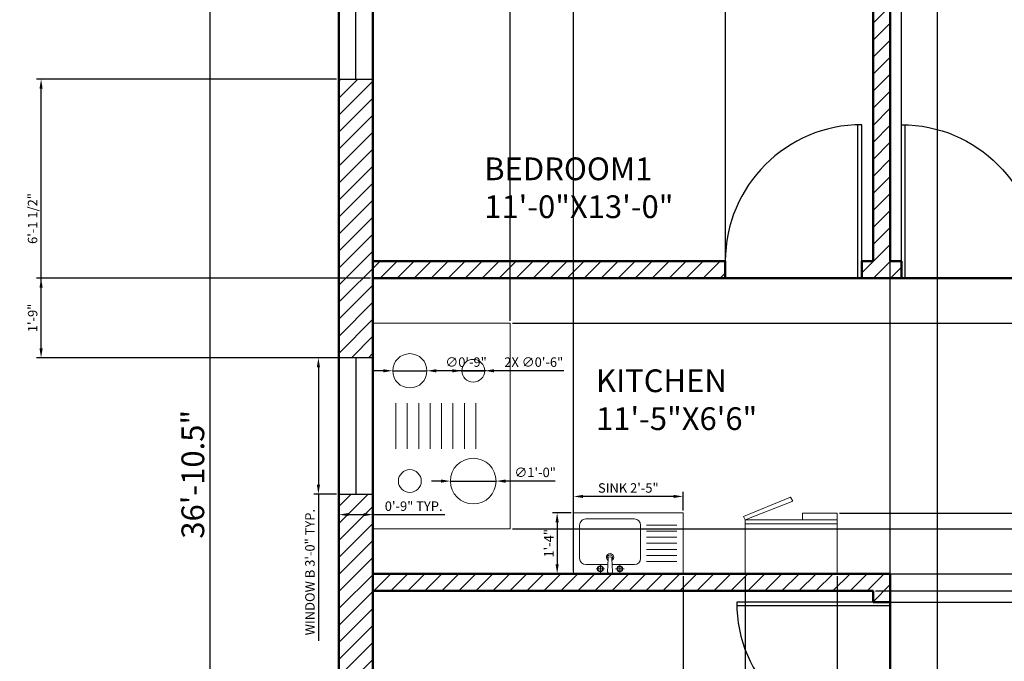
# Model space of a CAD drawing. Units: inches. Extents: x 3064 to 3516, y 2736 to 3280.
# Tile 3 of 5: x 3064 to 3324, y 2941 to 3110. Entities that reach past the tile are written whole.
import ezdxf

# ---------------------------------------------------------------- set-up
doc = ezdxf.new("R2010")
doc.units = ezdxf.units.IN
for name, color, linetype, lineweight in [('A-ANNO-DIMS', 2, 'Continuous', 18), ('A-AREA-IDEN', 6, 'Continuous', 25), ('A-DOOR', 3, 'Continuous', 25), ('A-EQPM', 8, 'Continuous', 18), ('A-FLOR-FIXT', 9, 'Continuous', 20), ('A-GLAZ', 5, 'Continuous', 25), ('A-WALL', 7, 'Continuous', 50), ('A-WALL-PATT', 8, 'Continuous', 13)]:
    doc.layers.add(name, color=color, linetype=linetype, lineweight=lineweight)
doc.styles.get("Standard").update_dxf_attribs({"font": 'arial.ttf'})
doc.dimstyles.new('ISO-25', dxfattribs={"dimtxt": 2.5, "dimasz": 2.5, "dimexe": 1.25, "dimexo": 0.625, "dimtad": 1, "dimlunit": 3, "dimtxsty": 'Standard', "dimcen": 2.5, "dimadec": 0, "dimazin": 0, "dimtfac": 1, "dimtmove": 0, "dimatfit": 3, "dimfxl": 1, "dimarcsym": 0})

# ---------------------------------------------------------------- blocks, each defined once
blk = doc.blocks.new('*D4')
at = {"layer": 'A-ANNO-DIMS', "color": 0, "lineweight": -2, "transparency": 16777216}
for p, q in [((3147.27, 3211.51), (3112.57, 3211.51)), ((3113.82, 3209.01), (3113.82, 2771.51)), ((3147.27, 2769.01), (3112.57, 2769.01))]:
    blk.add_line(p, q, dxfattribs=at)
at = {"layer": 'A-ANNO-DIMS', "color": 0, "transparency": 16777216}
for points in [[(3113.4, 3209.01), (3114.23, 3209.01), (3113.82, 3211.51)], [(3113.4, 2771.51), (3114.23, 2771.51), (3113.82, 2769.01)]]:
    blk.add_solid(points, dxfattribs=at)
at = {"layer": 'Defpoints', "color": 0, "transparency": 16777216}
for p in [(3147.9, 3211.51), (3113.82, 2769.01), (3147.9, 2769.01)]:
    blk.add_point(p, dxfattribs=at)
at = {"layer": 'A-ANNO-DIMS', "color": 0, "transparency": 16777216, "insert": (3110.13, 2990.26), "char_height": 6, "attachment_point": 5, "rotation": 90}
blk.add_mtext('36\'-10.5"', dxfattribs=at)
blk = doc.blocks.new('kitchen sink8')
at = {"color": 0}
for p, q in [((0, 0), (-1080, 0)), ((-1080, 0), (-1080, -600)), ((0, -600), (0, 0)), ((-379.8, -90), (-600, -90)), ((-498, -48), (-414, -48)), ((-456, -6), (-456, -90)), ((-377.9, -151.2), (-384.1, -17.1)), ((-335.9, -17.1), (-342.1, -151.2)), ((-120, -90), (-340.2, -90)), ((-222, -48), (-306, -48)), ((-264, -6), (-264, -90)), ((-1020, -120), (-720, -120)), ((-1020, -180), (-720, -180)), ((-660, -150), (-660, -480)), ((-60, -480), (-60, -150)), ((-1020, -240), (-720, -240)), ((-1020, -300), (-720, -300)), ((-1020, -360), (-720, -360)), ((-1020, -420), (-720, -420)), ((-1020, -480), (-720, -480)), ((-600, -540), (-120, -540)), ((-1080, -600), (0, -600))]:
    blk.add_line(p, q, dxfattribs=at)
for centre, radius in [((-456, -48), 30), ((-456, -48), 24), ((-264, -48), 30), ((-264, -48), 24)]:
    blk.add_circle(centre, radius, dxfattribs=at)
for centre, radius, start, end in [((-360, -25.5), 25.5, 19.33284, 160.66716), ((-600, -150), 60, 90, 180), ((-120, -150), 60, 0, 90), ((-360, -162), 36, 121.86593, 58.13407), ((-360, -162), 24, 139.21522, 40.78479), ((-360, -149.3), 18, 186.0661, 353.9339), ((-600, -480), 60, 180, 270), ((-120, -480), 60, 270, 0)]:
    blk.add_arc(centre, radius, start, end, dxfattribs=at)
blk = doc.blocks.new('DOOR-SWING-36IN')
for p, q in [((-1, -4.5), (-1, 36)), ((0, 0), (0, 36))]:
    blk.add_line(p, q)
blk.add_arc((0, 0), 36, 90, 180)
blk = doc.blocks.new('WIN-60IN')
for p, q in [((0, 60), (0, 0)), ((9, 60), (0, 60)), ((4.5, 60), (4.5, 0)), ((9, 0), (9, 60)), ((0, 0), (9, 0))]:
    blk.add_line(p, q)
blk = doc.blocks.new('WIN-36IN')
for p, q in [((36, 9), (0, 9)), ((0, 9), (0, 0)), ((36, 0), (36, 9)), ((0, 4.5), (36, 4.5)), ((0, 0), (36, 0))]:
    blk.add_line(p, q)
blk = doc.blocks.new('*D21')
at = {"layer": 'A-ANNO-DIMS', "color": 0, "lineweight": -2, "transparency": 16777216}
for p, q in [((3147.27, 3021.01), (3141.25, 3021.01)), ((3142.5, 3018.51), (3142.5, 2987.51)), ((3147.27, 2985.01), (3141.25, 2985.01)), ((3142.5, 2985.01), (3142.5, 2946.33))]:
    blk.add_line(p, q, dxfattribs=at)
at = {"layer": 'A-ANNO-DIMS', "color": 0, "transparency": 16777216}
for points in [[(3142.08, 3018.51), (3142.91, 3018.51), (3142.5, 3021.01)], [(3142.08, 2987.51), (3142.91, 2987.51), (3142.5, 2985.01)]]:
    blk.add_solid(points, dxfattribs=at)
at = {"layer": 'Defpoints', "color": 0, "transparency": 16777216}
for p in [(3147.9, 3021.01), (3142.5, 2985.01), (3147.9, 2985.01)]:
    blk.add_point(p, dxfattribs=at)
at = {"layer": 'A-ANNO-DIMS', "color": 0, "transparency": 16777216, "insert": (3140.58, 2964.42), "char_height": 2.5, "attachment_point": 5, "rotation": 90}
blk.add_mtext('WINDOW B 3\'-0" TYP.', dxfattribs=at)
blk = doc.blocks.new('*D22')
at = {"layer": 'A-ANNO-DIMS', "color": 0, "lineweight": -2, "transparency": 16777216}
for p, q in [((3147.9, 2984.39), (3147.9, 2978.36)), ((3156.9, 2984.39), (3156.9, 2978.36)), ((3150.4, 2979.61), (3154.4, 2979.61)), ((3156.9, 2979.61), (3175.89, 2979.61))]:
    blk.add_line(p, q, dxfattribs=at)
at = {"layer": 'A-ANNO-DIMS', "color": 0, "transparency": 16777216}
for points in [[(3150.4, 2980.03), (3150.4, 2979.2), (3147.9, 2979.61)], [(3154.4, 2980.03), (3154.4, 2979.2), (3156.9, 2979.61)]]:
    blk.add_solid(points, dxfattribs=at)
at = {"layer": 'Defpoints', "color": 0, "transparency": 16777216}
for p in [(3147.9, 2985.01), (3156.9, 2985.01), (3156.9, 2979.61)]:
    blk.add_point(p, dxfattribs=at)
at = {"layer": 'A-ANNO-DIMS', "color": 0, "transparency": 16777216, "insert": (3167.64, 2981.52), "char_height": 2.5, "attachment_point": 5}
blk.add_mtext('0\'-9" TYP.', dxfattribs=at)
blk = doc.blocks.new('*D33')
at = {"layer": 'A-ANNO-DIMS', "color": 0, "lineweight": -2, "transparency": 16777216}
for p, q in [((3209.84, 2980.7), (3209.84, 2985.66)), ((3236.24, 2984.41), (3212.34, 2984.41)), ((3238.74, 2980.7), (3238.74, 2985.66))]:
    blk.add_line(p, q, dxfattribs=at)
at = {"layer": 'A-ANNO-DIMS', "color": 0, "transparency": 16777216}
for points in [[(3212.34, 2984.82), (3212.34, 2983.99), (3209.84, 2984.41)], [(3236.24, 2984.82), (3236.24, 2983.99), (3238.74, 2984.41)]]:
    blk.add_solid(points, dxfattribs=at)
at = {"layer": 'Defpoints', "color": 0, "transparency": 16777216}
for p in [(3209.84, 2984.41), (3209.84, 2980.07), (3238.74, 2980.07)]:
    blk.add_point(p, dxfattribs=at)
at = {"layer": 'A-ANNO-DIMS', "color": 0, "transparency": 16777216, "insert": (3224.29, 2986.32), "char_height": 2.5, "attachment_point": 5}
blk.add_mtext('SINK 2\'-5"', dxfattribs=at)
blk = doc.blocks.new('*D34')
at = {"layer": 'A-ANNO-DIMS', "color": 0, "lineweight": -2, "transparency": 16777216}
for p, q in [((3209.22, 2980.07), (3204.26, 2980.07)), ((3205.51, 2977.57), (3205.51, 2966.51)), ((3209.22, 2964.01), (3204.26, 2964.01))]:
    blk.add_line(p, q, dxfattribs=at)
at = {"layer": 'A-ANNO-DIMS', "color": 0, "transparency": 16777216}
for points in [[(3205.09, 2977.57), (3205.92, 2977.57), (3205.51, 2980.07)], [(3205.09, 2966.51), (3205.92, 2966.51), (3205.51, 2964.01)]]:
    blk.add_solid(points, dxfattribs=at)
at = {"layer": 'Defpoints', "color": 0, "transparency": 16777216}
for p in [(3209.84, 2980.07), (3205.51, 2964.01), (3209.84, 2964.01)]:
    blk.add_point(p, dxfattribs=at)
at = {"layer": 'A-ANNO-DIMS', "color": 0, "transparency": 16777216, "insert": (3203.63, 2972.04), "char_height": 2.5, "attachment_point": 5, "rotation": 90}
blk.add_mtext('1\'-4"', dxfattribs=at)
blk = doc.blocks.new('*D39')
at = {"layer": 'A-ANNO-DIMS', "color": 0, "lineweight": -2, "transparency": 16777216}
for p, q in [((3156.27, 3042.01), (3068.05, 3042.01)), ((3069.3, 3023.51), (3069.3, 3039.51)), ((3156.27, 3021.01), (3068.05, 3021.01))]:
    blk.add_line(p, q, dxfattribs=at)
at = {"layer": 'A-ANNO-DIMS', "color": 0, "transparency": 16777216}
for points in [[(3068.88, 3039.51), (3069.71, 3039.51), (3069.3, 3042.01)], [(3068.88, 3023.51), (3069.71, 3023.51), (3069.3, 3021.01)]]:
    blk.add_solid(points, dxfattribs=at)
at = {"layer": 'Defpoints', "color": 0, "transparency": 16777216}
for p in [(3069.3, 3042.01), (3156.9, 3042.01), (3156.9, 3021.01)]:
    blk.add_point(p, dxfattribs=at)
at = {"layer": 'A-ANNO-DIMS', "color": 0, "transparency": 16777216, "insert": (3067.4, 3031.51), "char_height": 2.5, "attachment_point": 5, "rotation": 90}
blk.add_mtext('1\'-9"', dxfattribs=at)
blk = doc.blocks.new('*D40')
at = {"layer": 'A-ANNO-DIMS', "color": 0, "lineweight": -2, "transparency": 16777216}
for p, q in [((3147.27, 3094.51), (3068.05, 3094.51)), ((3069.3, 3023.51), (3069.3, 3092.01)), ((3147.27, 3021.01), (3068.05, 3021.01))]:
    blk.add_line(p, q, dxfattribs=at)
at = {"layer": 'A-ANNO-DIMS', "color": 0, "transparency": 16777216}
for points in [[(3068.88, 3092.01), (3069.71, 3092.01), (3069.3, 3094.51)], [(3068.88, 3023.51), (3069.71, 3023.51), (3069.3, 3021.01)]]:
    blk.add_solid(points, dxfattribs=at)
at = {"layer": 'Defpoints', "color": 0, "transparency": 16777216}
for p in [(3069.3, 3094.51), (3147.9, 3094.51), (3147.9, 3021.01)]:
    blk.add_point(p, dxfattribs=at)
at = {"layer": 'A-ANNO-DIMS', "color": 0, "transparency": 16777216, "insert": (3067.38, 3057.76), "char_height": 2.5, "attachment_point": 5, "rotation": 90}
blk.add_mtext('6\'-1 1/2"', dxfattribs=at)
blk = doc.blocks.new('*D50')
at = {"layer": 'A-ANNO-DIMS', "color": 0, "lineweight": -2, "transparency": 16777216}
for p, q in [((3156.9, 3030.78), (3156.9, 3240.36)), ((3159.4, 3239.11), (3190.59, 3239.11)), ((3193.09, 3030.78), (3193.09, 3240.36))]:
    blk.add_line(p, q, dxfattribs=at)
at = {"layer": 'A-ANNO-DIMS', "color": 0, "transparency": 16777216}
for points in [[(3159.4, 3239.53), (3159.4, 3238.7), (3156.9, 3239.11)], [(3190.59, 3239.53), (3190.59, 3238.7), (3193.09, 3239.11)]]:
    blk.add_solid(points, dxfattribs=at)
at = {"layer": 'Defpoints', "color": 0, "transparency": 16777216}
for p in [(3193.09, 3239.11), (3156.9, 3030.16), (3193.09, 3030.16)]:
    blk.add_point(p, dxfattribs=at)
at = {"layer": 'A-ANNO-DIMS', "color": 0, "transparency": 16777216, "insert": (3174.99, 3241.02), "char_height": 2.5, "attachment_point": 5}
blk.add_mtext('3\'-0"', dxfattribs=at)
blk = doc.blocks.new('*D51')
at = {"layer": 'A-ANNO-DIMS', "color": 0, "lineweight": -2, "transparency": 16777216}
for p, q in [((3193.71, 3030.16), (3515.25, 3030.16)), ((3514, 3027.66), (3514, 2978.37)), ((3193.71, 2975.87), (3515.25, 2975.87))]:
    blk.add_line(p, q, dxfattribs=at)
at = {"layer": 'A-ANNO-DIMS', "color": 0, "transparency": 16777216}
for points in [[(3513.58, 3027.66), (3514.41, 3027.66), (3514, 3030.16)], [(3513.58, 2978.37), (3514.41, 2978.37), (3514, 2975.87)]]:
    blk.add_solid(points, dxfattribs=at)
at = {"layer": 'Defpoints', "color": 0, "transparency": 16777216}
for p in [(3193.09, 3030.16), (3193.09, 2975.87), (3514, 2975.87)]:
    blk.add_point(p, dxfattribs=at)
at = {"layer": 'A-ANNO-DIMS', "color": 0, "transparency": 16777216, "insert": (3512.08, 3003.01), "char_height": 2.5, "attachment_point": 5, "rotation": 90}
blk.add_mtext('4\'-6 1/2"', dxfattribs=at)
blk = doc.blocks.new('*D52')
at = {"layer": 'A-ANNO-DIMS', "color": 0, "lineweight": -2, "transparency": 16777216}
for p, q in [((3156.9, 2964.64), (3156.9, 3240.36)), ((3159.4, 3239.11), (3207.34, 3239.11)), ((3209.84, 2964.64), (3209.84, 3240.36))]:
    blk.add_line(p, q, dxfattribs=at)
at = {"layer": 'A-ANNO-DIMS', "color": 0, "transparency": 16777216}
for points in [[(3159.4, 3239.53), (3159.4, 3238.7), (3156.9, 3239.11)], [(3207.34, 3239.53), (3207.34, 3238.7), (3209.84, 3239.11)]]:
    blk.add_solid(points, dxfattribs=at)
at = {"layer": 'Defpoints', "color": 0, "transparency": 16777216}
for p in [(3209.84, 3239.11), (3156.9, 2964.01), (3209.84, 2964.01)]:
    blk.add_point(p, dxfattribs=at)
at = {"layer": 'A-ANNO-DIMS', "color": 0, "transparency": 16777216, "insert": (3183.37, 3241.01), "char_height": 2.5, "attachment_point": 5}
blk.add_mtext('4\'-5"', dxfattribs=at)
blk = doc.blocks.new('*D53')
at = {"layer": 'A-ANNO-DIMS', "color": 0, "lineweight": -2, "transparency": 16777216}
for p, q in [((3238.74, 2963.39), (3238.74, 2740.16)), ((3255.12, 2963.39), (3255.12, 2740.16)), ((3241.24, 2741.41), (3252.62, 2741.41))]:
    blk.add_line(p, q, dxfattribs=at)
at = {"layer": 'A-ANNO-DIMS', "color": 0, "transparency": 16777216}
for points in [[(3241.24, 2741.83), (3241.24, 2741), (3238.74, 2741.41)], [(3252.62, 2741.83), (3252.62, 2741), (3255.12, 2741.41)]]:
    blk.add_solid(points, dxfattribs=at)
at = {"layer": 'Defpoints', "color": 0, "transparency": 16777216}
for p in [(3238.74, 2964.01), (3255.12, 2964.01), (3255.12, 2741.41)]:
    blk.add_point(p, dxfattribs=at)
at = {"layer": 'A-ANNO-DIMS', "color": 0, "transparency": 16777216, "insert": (3246.93, 2743.33), "char_height": 2.5, "attachment_point": 5}
blk.add_mtext('1\'-4 1/2"', dxfattribs=at)
blk = doc.blocks.new('*D54')
at = {"layer": 'A-ANNO-DIMS', "color": 0, "lineweight": -2, "transparency": 16777216}
for p, q in [((3255.12, 2963.39), (3255.12, 2740.16)), ((3279.41, 2963.39), (3279.41, 2740.16)), ((3257.62, 2741.41), (3276.91, 2741.41))]:
    blk.add_line(p, q, dxfattribs=at)
at = {"layer": 'A-ANNO-DIMS', "color": 0, "transparency": 16777216}
for points in [[(3257.62, 2741.83), (3257.62, 2741), (3255.12, 2741.41)], [(3276.91, 2741.83), (3276.91, 2741), (3279.41, 2741.41)]]:
    blk.add_solid(points, dxfattribs=at)
at = {"layer": 'Defpoints', "color": 0, "transparency": 16777216}
for p in [(3255.12, 2964.01), (3279.41, 2964.01), (3279.41, 2741.41)]:
    blk.add_point(p, dxfattribs=at)
at = {"layer": 'A-ANNO-DIMS', "color": 0, "transparency": 16777216, "insert": (3267.26, 2743.33), "char_height": 2.5, "attachment_point": 5}
blk.add_mtext('2\'-0 1/2"', dxfattribs=at)
blk = doc.blocks.new('*D55')
at = {"layer": 'A-ANNO-DIMS', "color": 0, "lineweight": -2, "transparency": 16777216}
for p, q in [((3280.03, 2979.98), (3515.25, 2979.98)), ((3514, 2966.51), (3514, 2977.48)), ((3280.03, 2964.01), (3515.25, 2964.01))]:
    blk.add_line(p, q, dxfattribs=at)
at = {"layer": 'A-ANNO-DIMS', "color": 0, "transparency": 16777216}
for points in [[(3513.58, 2977.48), (3514.41, 2977.48), (3514, 2979.98)], [(3513.58, 2966.51), (3514.41, 2966.51), (3514, 2964.01)]]:
    blk.add_solid(points, dxfattribs=at)
at = {"layer": 'Defpoints', "color": 0, "transparency": 16777216}
for p in [(3279.41, 2979.98), (3514, 2979.98), (3279.41, 2964.01)]:
    blk.add_point(p, dxfattribs=at)
at = {"layer": 'A-ANNO-DIMS', "color": 0, "transparency": 16777216, "insert": (3512.12, 2972), "char_height": 2.5, "attachment_point": 5, "rotation": 90}
blk.add_mtext('1\'-4"', dxfattribs=at)
blk = doc.blocks.new('*D56')
at = {"layer": 'A-ANNO-DIMS', "color": 0, "lineweight": -2, "transparency": 16777216}
for p, q in [((3157.52, 3042.01), (3515.25, 3042.01)), ((3514, 3032.66), (3514, 3039.51)), ((3193.71, 3030.16), (3515.25, 3030.16))]:
    blk.add_line(p, q, dxfattribs=at)
at = {"layer": 'A-ANNO-DIMS', "color": 0, "transparency": 16777216}
for points in [[(3513.58, 3039.51), (3514.41, 3039.51), (3514, 3042.01)], [(3513.58, 3032.66), (3514.41, 3032.66), (3514, 3030.16)]]:
    blk.add_solid(points, dxfattribs=at)
at = {"layer": 'Defpoints', "color": 0, "transparency": 16777216}
for p in [(3156.9, 3042.01), (3514, 3042.01), (3193.09, 3030.16)]:
    blk.add_point(p, dxfattribs=at)
at = {"layer": 'A-ANNO-DIMS', "color": 0, "transparency": 16777216, "insert": (3512.1, 3036.09), "char_height": 2.5, "attachment_point": 5, "rotation": 90}
blk.add_mtext('1\'-0"', dxfattribs=at)
blk = doc.blocks.new('*D57')
at = {"layer": 'A-ANNO-DIMS', "color": 0, "lineweight": -2, "transparency": 16777216}
for p, q in [((3156.9, 3047.14), (3156.9, 3240.36)), ((3159.4, 3239.11), (3247.4, 3239.11)), ((3249.9, 3047.14), (3249.9, 3240.36))]:
    blk.add_line(p, q, dxfattribs=at)
at = {"layer": 'A-ANNO-DIMS', "color": 0, "transparency": 16777216}
for points in [[(3159.4, 3239.53), (3159.4, 3238.7), (3156.9, 3239.11)], [(3247.4, 3239.53), (3247.4, 3238.7), (3249.9, 3239.11)]]:
    blk.add_solid(points, dxfattribs=at)
at = {"layer": 'Defpoints', "color": 0, "transparency": 16777216}
for p in [(3249.9, 3239.11), (3156.9, 3046.51), (3249.9, 3046.51)]:
    blk.add_point(p, dxfattribs=at)
at = {"layer": 'A-ANNO-DIMS', "color": 0, "transparency": 16777216, "insert": (3203.4, 3241.02), "char_height": 2.5, "attachment_point": 5}
blk.add_mtext('7\'-9"', dxfattribs=at)
blk = doc.blocks.new('*D59')
at = {"layer": 'A-ANNO-DIMS', "color": 0, "lineweight": -2, "transparency": 16777216}
for p, q in [((3514, 2962.01), (3514, 2972.41)), ((3289.52, 2959.51), (3515.25, 2959.51)), ((3514, 2956.51), (3514, 2959.51)), ((3289.52, 2956.51), (3515.25, 2956.51)), ((3514, 2954.01), (3514, 2951.51))]:
    blk.add_line(p, q, dxfattribs=at)
at = {"layer": 'A-ANNO-DIMS', "color": 0, "transparency": 16777216}
for points in [[(3513.58, 2962.01), (3514.41, 2962.01), (3514, 2959.51)], [(3513.58, 2954.01), (3514.41, 2954.01), (3514, 2956.51)]]:
    blk.add_solid(points, dxfattribs=at)
at = {"layer": 'Defpoints', "color": 0, "transparency": 16777216}
for p in [(3288.9, 2959.51), (3514, 2959.51), (3288.9, 2956.51)]:
    blk.add_point(p, dxfattribs=at)
at = {"layer": 'A-ANNO-DIMS', "color": 0, "transparency": 16777216, "insert": (3512.09, 2968.46), "char_height": 2.5, "attachment_point": 5, "rotation": 90}
blk.add_mtext('0\'-3"', dxfattribs=at)
blk = doc.blocks.new('*D61')
at = {"layer": 'A-ANNO-DIMS', "color": 0, "lineweight": -2, "transparency": 16777216}
for p, q in [((3293.4, 2861.14), (3293.4, 3240.36)), ((3295.9, 3239.11), (3303.4, 3239.11)), ((3305.9, 2861.14), (3305.9, 3240.36)), ((3305.9, 3239.11), (3321.88, 3239.11))]:
    blk.add_line(p, q, dxfattribs=at)
at = {"layer": 'A-ANNO-DIMS', "color": 0, "transparency": 16777216}
for points in [[(3295.9, 3239.53), (3295.9, 3238.7), (3293.4, 3239.11)], [(3303.4, 3239.53), (3303.4, 3238.7), (3305.9, 3239.11)]]:
    blk.add_solid(points, dxfattribs=at)
at = {"layer": 'Defpoints', "color": 0, "transparency": 16777216}
for p in [(3305.9, 3239.11), (3293.4, 2860.51), (3305.9, 2860.51)]:
    blk.add_point(p, dxfattribs=at)
at = {"layer": 'A-ANNO-DIMS', "color": 0, "transparency": 16777216, "insert": (3315.14, 3241.03), "char_height": 2.5, "attachment_point": 5}
blk.add_mtext('1\'-0 1/2"', dxfattribs=at)
blk = doc.blocks.new('*D62')
at = {"layer": 'A-ANNO-DIMS', "color": 0, "lineweight": -2, "transparency": 16777216}
for p, q in [((3290.9, 3239.11), (3288.4, 3239.11)), ((3293.4, 3047.14), (3293.4, 3240.36)), ((3293.4, 3239.11), (3296.4, 3239.11)), ((3296.4, 3047.14), (3296.4, 3240.36)), ((3298.9, 3239.11), (3309.29, 3239.11))]:
    blk.add_line(p, q, dxfattribs=at)
at = {"layer": 'A-ANNO-DIMS', "color": 0, "transparency": 16777216}
for points in [[(3290.9, 3239.53), (3290.9, 3238.7), (3293.4, 3239.11)], [(3298.9, 3239.53), (3298.9, 3238.7), (3296.4, 3239.11)]]:
    blk.add_solid(points, dxfattribs=at)
at = {"layer": 'Defpoints', "color": 0, "transparency": 16777216}
for p in [(3296.4, 3239.11), (3293.4, 3046.51), (3296.4, 3046.51)]:
    blk.add_point(p, dxfattribs=at)
at = {"layer": 'A-ANNO-DIMS', "color": 0, "transparency": 16777216, "insert": (3305.35, 3241.02), "char_height": 2.5, "attachment_point": 5}
blk.add_mtext('0\'-3"', dxfattribs=at)
blk = doc.blocks.new('*D64')
at = {"layer": 'A-ANNO-DIMS', "color": 0, "lineweight": -2, "transparency": 16777216}
for p, q in [((3159.6, 3017.57), (3157.1, 3017.57)), ((3162.1, 3017.57), (3171.15, 3017.57)), ((3186.77, 3017.57), (3173.65, 3017.57))]:
    blk.add_line(p, q, dxfattribs=at)
at = {"layer": 'A-ANNO-DIMS', "color": 0, "transparency": 16777216}
for points in [[(3159.6, 3017.99), (3159.6, 3017.15), (3162.1, 3017.57)], [(3173.65, 3017.99), (3173.65, 3017.15), (3171.15, 3017.57)]]:
    blk.add_solid(points, dxfattribs=at)
at = {"layer": 'Defpoints', "color": 0, "transparency": 16777216}
for p in [(3162.1, 3017.57), (3171.15, 3017.57)]:
    blk.add_point(p, dxfattribs=at)
at = {"layer": 'A-ANNO-DIMS', "color": 0, "transparency": 16777216, "insert": (3181.46, 3019.54), "char_height": 2.5, "attachment_point": 5, "rotation": 359.9955}
blk.add_mtext('∅0\'-9"', dxfattribs=at)
blk = doc.blocks.new('*D65')
at = {"layer": 'A-ANNO-DIMS', "color": 0, "lineweight": -2, "transparency": 16777216}
for p, q in [((3174.83, 2988.46), (3172.33, 2988.46)), ((3177.33, 2988.46), (3189.39, 2988.46)), ((3205.01, 2988.46), (3191.89, 2988.46))]:
    blk.add_line(p, q, dxfattribs=at)
at = {"layer": 'A-ANNO-DIMS', "color": 0, "transparency": 16777216}
for points in [[(3174.83, 2988.88), (3174.83, 2988.04), (3177.33, 2988.46)], [(3191.89, 2988.88), (3191.89, 2988.04), (3189.39, 2988.46)]]:
    blk.add_solid(points, dxfattribs=at)
at = {"layer": 'Defpoints', "color": 0, "transparency": 16777216}
for p in [(3177.33, 2988.46), (3189.39, 2988.46)]:
    blk.add_point(p, dxfattribs=at)
at = {"layer": 'A-ANNO-DIMS', "color": 0, "transparency": 16777216, "insert": (3199.7, 2990.43), "char_height": 2.5, "attachment_point": 5, "rotation": 0.0047}
blk.add_mtext('∅1\'-0"', dxfattribs=at)
blk = doc.blocks.new('*D66')
at = {"layer": 'A-ANNO-DIMS', "color": 0, "lineweight": -2, "transparency": 16777216}
for p, q in [((3177.85, 3017.57), (3175.35, 3017.57)), ((3180.35, 3017.57), (3186.38, 3017.57)), ((3207.27, 3017.57), (3188.88, 3017.57))]:
    blk.add_line(p, q, dxfattribs=at)
at = {"layer": 'A-ANNO-DIMS', "color": 0, "transparency": 16777216}
for points in [[(3177.85, 3017.98), (3177.85, 3017.15), (3180.35, 3017.57)], [(3188.88, 3017.99), (3188.88, 3017.15), (3186.38, 3017.57)]]:
    blk.add_solid(points, dxfattribs=at)
at = {"layer": 'Defpoints', "color": 0, "transparency": 16777216}
for p in [(3180.35, 3017.57), (3186.38, 3017.57)]:
    blk.add_point(p, dxfattribs=at)
at = {"layer": 'A-ANNO-DIMS', "color": 0, "transparency": 16777216, "insert": (3199.33, 3019.54), "char_height": 2.5, "attachment_point": 5, "rotation": 0.0122}
blk.add_mtext('2X ∅0\'-6"', dxfattribs=at)

msp = doc.modelspace()

# ---------------------------------------------------------------- hatches: boundary and pattern name
at = {"layer": 'A-WALL-PATT'}
h = msp.add_hatch(dxfattribs=at)
h.set_pattern_fill('ANSI31', color=256)
h.paths.add_polyline_path([(3156.897, 2985.015), (3147.897, 2985.015), (3147.897, 2923.515), (3156.897, 2923.515)])
h.paths.add_polyline_path([(3156.897, 2863.515), (3147.897, 2863.515), (3147.897, 2812.515), (3156.897, 2812.515)])
h.paths.add_polyline_path([(3293.397, 2778.015), (3239.397, 2778.015), (3239.397, 2780.015), (3234.897, 2780.015), (3234.897, 2778.015), (3156.897, 2778.015), (3156.897, 2788.515), (3147.897, 2788.515), (3147.897, 2769.015), (3293.397, 2769.015)])
h.paths.add_polyline_path([(3369.397, 2778.015), (3343.897, 2778.015), (3344.15, 2769.015), (3369.397, 2769.015)])
h.paths.add_polyline_path([(3435.397, 2788.515), (3426.397, 2788.515), (3426.397, 2778.015), (3405.397, 2778.015), (3405.397, 2769.015), (3435.397, 2769.015)])
h.paths.add_polyline_path([(3435.397, 2960.265), (3426.397, 2960.265), (3426.397, 2812.515), (3435.397, 2812.515)])
h.paths.add_polyline_path([(3435.397, 3094.515), (3426.397, 3094.515), (3426.397, 3020.265), (3435.397, 3020.265)])
h.paths.add_polyline_path([(3435.397, 3211.515), (3147.897, 3211.515), (3147.897, 3154.515), (3156.897, 3154.515), (3156.897, 3202.515), (3426.397, 3202.515), (3426.397, 3154.515), (3435.397, 3154.515)])
h.paths.add_polyline_path([(3293.397, 3202.515), (3288.897, 3202.515), (3288.897, 3046.515), (3285.897, 3046.515), (3285.897, 3042.015), (3296.397, 3042.015), (3296.397, 3046.515), (3293.397, 3046.515)])
h.paths.add_polyline_path([(3426.397, 3046.515), (3332.397, 3046.515), (3332.397, 3042.015), (3426.397, 3042.015)])
h.paths.add_polyline_path([(3249.897, 3046.515), (3156.897, 3046.515), (3156.897, 3042.015), (3249.897, 3042.015)])
h.paths.add_polyline_path([(3156.897, 3094.515), (3147.897, 3094.515), (3147.897, 3021.015), (3156.897, 3021.015)])
h.paths.add_polyline_path([(3293.397, 2964.015), (3156.897, 2964.015), (3156.897, 2959.515), (3288.897, 2959.515), (3288.897, 2956.515), (3293.397, 2956.515)])
h.paths.add_polyline_path([(3249.897, 2827.515), (3156.897, 2827.515), (3156.897, 2823.015), (3234.897, 2823.015), (3234.897, 2816.015), (3239.397, 2816.015), (3239.397, 2823.015), (3249.897, 2823.015)])
h.paths.add_polyline_path([(3293.397, 2920.515), (3288.897, 2920.515), (3288.897, 2827.515), (3285.897, 2827.515), (3285.897, 2823.015), (3293.397, 2823.015), (3293.397, 2856.015), (3305.897, 2856.015), (3305.897, 2860.515), (3293.397, 2860.515)])
h.paths.add_polyline_path([(3348.397, 2920.515), (3343.897, 2920.515), (3343.897, 2860.515), (3341.897, 2860.515), (3341.897, 2856.015), (3343.897, 2856.015), (3343.897, 2778.015), (3348.397, 2778.015), (3348.397, 2823.015), (3350.397, 2823.015), (3350.397, 2827.515), (3348.397, 2827.515)])
h.paths.add_polyline_path([(3426.397, 2827.515), (3386.397, 2827.515), (3386.397, 2823.015), (3426.397, 2823.015)])

# ---------------------------------------------------------------- linework, layer by layer
at = {"layer": 'A-EQPM'}
for p, q in [((3162.929, 2996.983), (3162.929, 3009.047)), ((3165.945, 2996.983), (3165.945, 3009.047)), ((3168.961, 2996.983), (3168.961, 3009.047)), ((3171.978, 2996.983), (3171.978, 3009.047)), ((3174.994, 2996.983), (3174.994, 3009.047)), ((3178.01, 2996.983), (3178.01, 3009.047)), ((3181.026, 2996.983), (3181.026, 3009.047)), ((3184.042, 2996.983), (3184.042, 3009.047)), ((3267.122, 2984.207), (3254.664, 2979.092)), ((3267.738, 2983.14), (3267.122, 2984.207)), ((3255.121, 2978.257), (3267.738, 2983.14)), ((3254.664, 2979.092), (3255.146, 2978.257)), ((3279.406, 2978.257), (3255.121, 2978.257)), ((3255.121, 2978.257), (3255.121, 2964.015)), ((3279.406, 2979.978), (3270.277, 2979.978)), ((3270.277, 2979.978), (3270.277, 2978.257)), ((3279.406, 2978.257), (3279.406, 2979.978)), ((3279.406, 2964.015), (3279.406, 2978.257)), ((3255.121, 2977.149), (3279.406, 2977.149))]:
    msp.add_line(p, q, dxfattribs=at)
msp.add_lwpolyline([(3193.09, 2975.87), (3156.897, 2975.87), (3156.897, 3030.159), (3193.09, 3030.159)], close=True, dxfattribs=at)
for centre, radius in [((3166.626, 3017.569), 4.524), ((3183.361, 3017.569), 3.016), ((3183.361, 2988.461), 6.032), ((3166.626, 2988.461), 3.016)]:
    msp.add_circle(centre, radius, dxfattribs=at)
at = {"layer": 'A-WALL'}
for p, q in [((3147.897, 3211.515), (3147.897, 2769.015)), ((3156.897, 3202.515), (3156.897, 2778.015)), ((3288.897, 3202.515), (3288.897, 3046.515)), ((3293.397, 3202.515), (3293.397, 3046.515)), ((3156.897, 3046.515), (3249.897, 3046.515)), ((3249.897, 3042.015), (3249.897, 3046.515)), ((3285.897, 3046.515), (3285.897, 3042.015)), ((3285.897, 3046.515), (3288.897, 3046.515)), ((3293.397, 3046.515), (3296.397, 3046.515)), ((3293.397, 3046.515), (3293.397, 3046.515)), ((3296.397, 3046.515), (3296.397, 3042.015)), ((3156.897, 3042.015), (3426.397, 3042.015)), ((3156.897, 2964.015), (3293.397, 2964.015)), ((3293.397, 2964.015), (3293.397, 2860.515)), ((3156.897, 2959.515), (3288.897, 2959.515)), ((3288.897, 2959.515), (3288.897, 2956.515)), ((3288.897, 2956.515), (3293.397, 2956.515))]:
    msp.add_line(p, q, dxfattribs=at)

# ---------------------------------------------------------------- block references
at = {"layer": 'A-DOOR'}
msp.add_blockref('DOOR-SWING-36IN', (3285.897, 3046.515), dxfattribs=at)
at = {"layer": 'A-DOOR', "extrusion": (0, 0, -1), "zscale": -1}
msp.add_blockref('DOOR-SWING-36IN', (-3296.397, 3046.515), dxfattribs=at)
at = {"layer": 'A-DOOR', "rotation": 90.00000000000033}
msp.add_blockref('DOOR-SWING-36IN', (3288.897, 2956.515), dxfattribs=at)
at = {"layer": 'A-FLOR-FIXT', "xscale": 0.0267598929419882, "yscale": 0.0267598929419882, "zscale": 0.0267598929419882, "rotation": 180}
msp.add_blockref('kitchen sink8', (3209.842, 2964.015), dxfattribs=at)
at = {"layer": 'A-GLAZ'}
for name, p, rotation in [('WIN-60IN', (3156.897, 3154.515), 180), ('WIN-36IN', (3147.897, 3021.015), 269.9999999999956)]:
    msp.add_blockref(name, p, dxfattribs=dict(at, rotation=rotation))

# ---------------------------------------------------------------- texts
at = {"layer": 'A-AREA-IDEN', "char_height": 6, "attachment_point": 1}
for s, width, insert in [('BEDROOM1\\P11\'-0"X13\'-0"', 94.64208, (3186.261, 3073.873)), ('KITCHEN\\P11\'-5"X6\'6"', 30.25977, (3215.768, 3017.939))]:
    msp.add_mtext_dynamic_manual_height_columns(s, width=width, gutter_width=12.5, heights=[0], dxfattribs=dict(at, insert=insert))

# ---------------------------------------------------------------- dimensions: what is measured, and where the dimension line sits
at = {"layer": 'A-ANNO-DIMS'}
for base, p1, p2, picture, middle in [((3305.897, 3239.115), (3293.397, 2860.515), (3305.897, 2860.515), '*D61', (3315.14, 3241.033)), ((3193.09, 3239.115), (3156.897, 3030.159), (3193.09, 3030.159), '*D50', (3174.994, 3241.017)), ((3249.897, 3239.115), (3156.897, 3046.515), (3249.897, 3046.515), '*D57', (3203.397, 3241.016)), ((3209.842, 3239.115), (3156.897, 2964.015), (3209.842, 2964.015), '*D52', (3183.37, 3241.011)), ((3296.397, 3239.115), (3293.397, 3046.515), (3296.397, 3046.515), '*D62', (3305.345, 3241.017)), ((3255.121, 2741.415), (3238.743, 2964.015), (3255.121, 2964.015), '*D53', (3246.932, 2743.333)), ((3279.406, 2741.415), (3255.121, 2964.015), (3279.406, 2964.015), '*D54', (3267.263, 2743.333))]:
    dim = msp.add_linear_dim(base=base, p1=p1, p2=p2, dimstyle='ISO-25', override={"dimdec": 1, "dimlfac": 1, "dimrnd": 0, "dimzin": 1, "dimdsep": 46, "dimlunit": 4, "dimfrac": 2}, dxfattribs=at)
    dim.commit()
    dim.dimension.update_dxf_attribs({"geometry": picture, "text_midpoint": middle})
for base, p1, p2, angle, override, picture, middle in [((3113.817, 2769.015), (3147.897, 3211.515), (3147.897, 2769.015), 90, {"dimtxt": 6, "dimclrd": 0, "dimclre": 0, "dimclrt": 0}, '*D4', (3110.126, 2990.265)), ((3069.297, 3094.515), (3147.897, 3021.015), (3147.897, 3094.515), 90, {"dimdec": 1, "dimlfac": 1, "dimrnd": 0, "dimzin": 1, "dimdsep": 46, "dimlunit": 4, "dimfrac": 2}, '*D40', (3067.38, 3057.765)), ((3069.297, 3042.015), (3156.897, 3021.015), (3156.897, 3042.015), 90, {"dimdec": 1, "dimlfac": 1, "dimrnd": 0, "dimzin": 1, "dimdsep": 46, "dimlunit": 4, "dimfrac": 2}, '*D39', (3067.396, 3031.515)), ((3513.997, 3042.015), (3193.09, 3030.159), (3156.897, 3042.015), 90, {"dimdec": 1, "dimlfac": 1, "dimrnd": 0, "dimzin": 1, "dimdsep": 46, "dimlunit": 4, "dimfrac": 2}, '*D56', (3512.096, 3036.087)), ((3513.997, 2975.87), (3193.09, 3030.159), (3193.09, 2975.87), 90, {"dimdec": 1, "dimlfac": 1, "dimrnd": 0, "dimzin": 1, "dimdsep": 46, "dimlunit": 4, "dimfrac": 2}, '*D51', (3512.08, 3003.015)), ((3205.507, 2964.015), (3209.842, 2980.071), (3209.842, 2964.015), 270, {"dimdec": 1, "dimlfac": 1, "dimrnd": 0, "dimzin": 1, "dimdsep": 46, "dimlunit": 4, "dimfrac": 2}, '*D34', (3203.627, 2972.043)), ((3513.997, 2979.978), (3279.406, 2964.015), (3279.406, 2979.978), 90, {"dimdec": 1, "dimlfac": 1, "dimrnd": 0, "dimzin": 1, "dimdsep": 46, "dimlunit": 4, "dimfrac": 2}, '*D55', (3512.117, 2971.997)), ((3513.997, 2959.515), (3288.897, 2956.515), (3288.897, 2959.515), 90, {"dimdec": 1, "dimlfac": 1, "dimrnd": 0, "dimzin": 1, "dimdsep": 46, "dimlunit": 4, "dimfrac": 2}, '*D59', (3512.095, 2968.463))]:
    dim = msp.add_linear_dim(base=base, p1=p1, p2=p2, angle=angle, dimstyle='ISO-25', override=override, dxfattribs=at)
    dim.commit()
    dim.dimension.update_dxf_attribs({"geometry": picture, "text_midpoint": middle})
dim = msp.add_diameter_dim_2p(p1=(3180.345, 3017.569), p2=(3186.377, 3017.57), text='2X <>', dimstyle='ISO-25', override={"dimdec": 1, "dimlfac": 1, "dimrnd": 0, "dimzin": 1, "dimdsep": 46, "dimlunit": 4, "dimfrac": 2}, dxfattribs=at)
dim.commit()
dim.dimension.update_dxf_attribs({"geometry": '*D66', "text_midpoint": (3199.326, 3017.573), "dimtype": 163})
for base, p1, p2, angle, text, picture, middle in [((3142.497, 2985.015), (3147.897, 3021.015), (3147.897, 2985.015), 270, 'WINDOW B <> TYP.', '*D21', (3140.578, 2964.422)), ((3209.842, 2984.406), (3238.743, 2980.071), (3209.842, 2980.071), 180, 'SINK <>', '*D33', (3224.292, 2986.324))]:
    dim = msp.add_linear_dim(base=base, p1=p1, p2=p2, angle=angle, text=text, dimstyle='ISO-25', override={"dimdec": 1, "dimlfac": 1, "dimrnd": 0, "dimzin": 1, "dimdsep": 46, "dimlunit": 4, "dimfrac": 2}, dxfattribs=at)
    dim.commit()
    dim.dimension.update_dxf_attribs({"geometry": picture, "text_midpoint": middle})
for p1, p2, picture, middle in [((3162.102, 3017.57), (3171.15, 3017.569), '*D64', (3181.458, 3017.568)), ((3177.329, 2988.46), (3189.393, 2988.461), '*D65', (3199.701, 2988.462))]:
    dim = msp.add_diameter_dim_2p(p1=p1, p2=p2, dimstyle='ISO-25', override={"dimdec": 1, "dimlfac": 1, "dimrnd": 0, "dimzin": 1, "dimdsep": 46, "dimlunit": 4, "dimfrac": 2}, dxfattribs=at)
    dim.commit()
    dim.dimension.update_dxf_attribs({"geometry": picture, "text_midpoint": middle})
dim = msp.add_linear_dim(base=(3156.897, 2979.615), p1=(3147.897, 2985.015), p2=(3156.897, 2985.015), text='<> TYP.', dimstyle='ISO-25', override={"dimdec": 1, "dimlfac": 1, "dimrnd": 0, "dimzin": 1, "dimdsep": 46, "dimlunit": 4, "dimfrac": 2}, dxfattribs=at)
dim.commit()
dim.dimension.update_dxf_attribs({"geometry": '*D22', "text_midpoint": (3167.642, 2981.516)})

doc.saveas('drawing.dxf')
